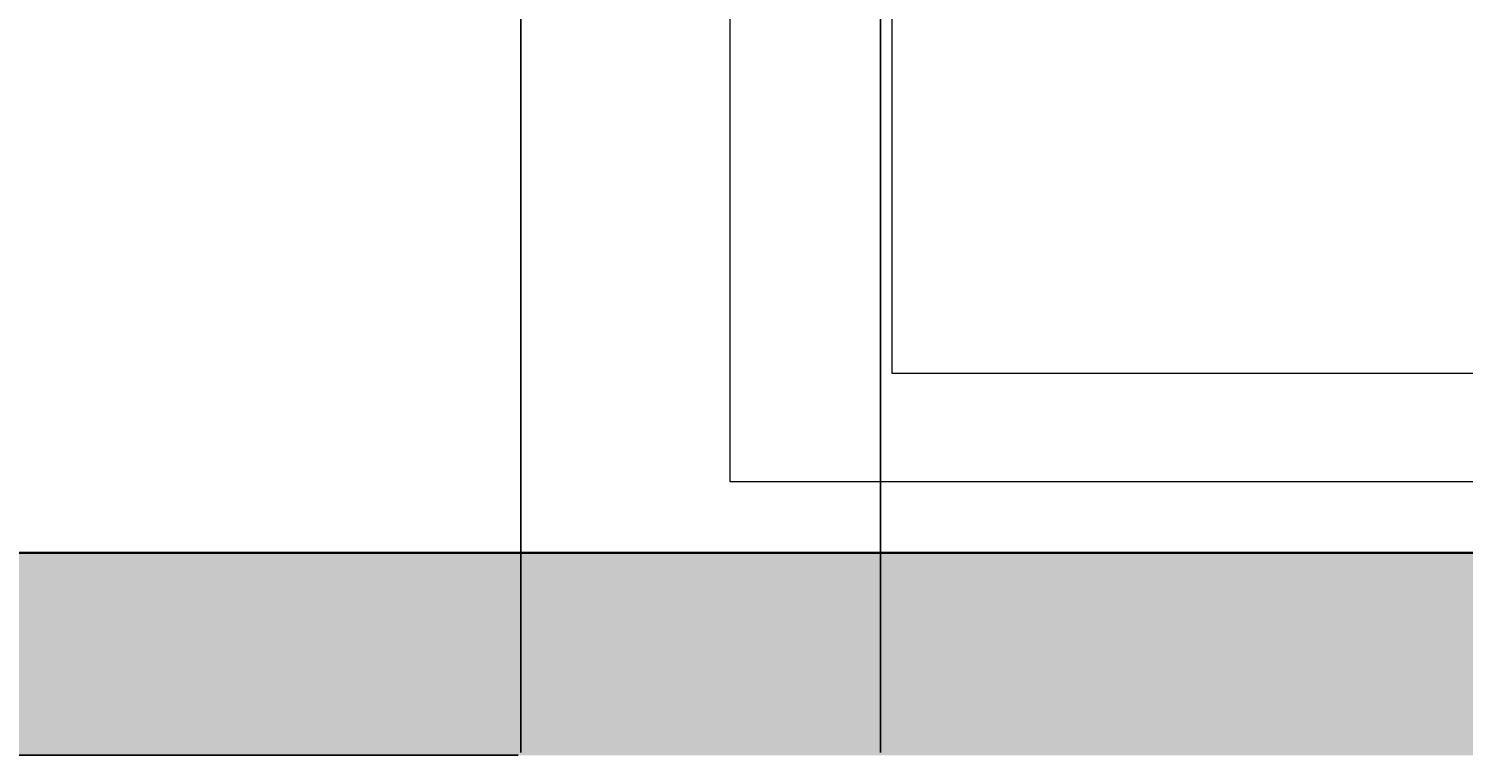
# Model space of a CAD drawing. Units: inches. Extents: x 1998 to 2588, y 1139 to 1977.
# Tile 123 of 134: x 2397 to 2429, y 1637 to 1653. Entities that reach past the tile are written whole.
import ezdxf

# ---------------------------------------------------------------- set-up
doc = ezdxf.new("R2010")
doc.units = ezdxf.units.IN
for name, color, linetype, lineweight in [('A-ANNO-DIMS', 2, 'Continuous', 18), ('A-WALL-PATT', 252, 'Continuous', 13), ('FUR', 21, 'Continuous', 18), ('WALL', 200, 'Continuous', 35)]:
    doc.layers.add(name, color=color, linetype=linetype, lineweight=lineweight)
doc.styles.get("Standard").update_dxf_attribs({"font": 'arial.ttf'})
doc.dimstyles.get("Standard").update_dxf_attribs({"dimtxt": 0.18, "dimasz": 0.18, "dimexe": 0.18, "dimexo": 0.0625, "dimgap": 0.09, "dimtad": 0, "dimtih": 1, "dimtoh": 1, "dimdec": 4, "dimzin": 0, "dimdsep": 46, "dimtxsty": 'Standard', "dimcen": 0.09, "dimadec": 0, "dimazin": 0, "dimtfac": 1, "dimtdec": 4, "dimtofl": 0, "dimtmove": 0, "dimatfit": 3, "dimfxl": 1, "dimtolj": 1, "dimtzin": 0, "dimarcsym": 0})

# ---------------------------------------------------------------- blocks, each defined once
blk = doc.blocks.new('SOFA-THREE-SEAT')
for p, q in [((0, 25.615), (0, 0)), ((0, 0), (74.336, 0))]:
    blk.add_line(p, q)
blk.add_lwpolyline([(3.604, 2.416), (71.008, 2.416), (71.008, 25.615), (3.604, 25.615)], close=True)
blk = doc.blocks.new('*D24')
at = {"layer": 'A-ANNO-DIMS', "color": 0, "lineweight": -2, "transparency": 16777216}
for p, q in [((2398.535, 1911.232), (2588.309, 1911.232)), ((2588.129, 1911.052), (2588.129, 1570.164)), ((2588.129, 1228.912), (2588.129, 1569.8)), ((2527.535, 1228.732), (2588.309, 1228.732))]:
    blk.add_line(p, q, dxfattribs=at)
at = {"layer": 'A-ANNO-DIMS', "color": 0, "transparency": 16777216}
for points in [[(2588.099, 1911.052), (2588.159, 1911.052), (2588.129, 1911.232)], [(2588.099, 1228.912), (2588.159, 1228.912), (2588.129, 1228.732)]]:
    blk.add_solid(points, dxfattribs=at)
at = {"layer": 'Defpoints', "color": 0, "transparency": 16777216}
for p in [(2398.473, 1911.232), (2588.129, 1911.232), (2527.473, 1228.732)]:
    blk.add_point(p, dxfattribs=at)
at = {"layer": 'A-ANNO-DIMS', "color": 0, "transparency": 16777216, "insert": (2588.129, 1569.982), "char_height": 0.18, "attachment_point": 5}
blk.add_mtext('\\A1;682.5', dxfattribs=at)
blk = doc.blocks.new('*D30')
at = {"layer": 'A-ANNO-DIMS', "color": 0, "lineweight": -2, "transparency": 16777216}
for p, q in [((2407.91, 1636.732), (1997.843, 1636.732)), ((1998.023, 1636.552), (1998.023, 1615.913)), ((1998.023, 1594.912), (1998.023, 1615.552)), ((2407.91, 1594.732), (1997.843, 1594.732))]:
    blk.add_line(p, q, dxfattribs=at)
at = {"layer": 'A-ANNO-DIMS', "color": 0, "transparency": 16777216}
for points in [[(1997.993, 1636.552), (1998.053, 1636.552), (1998.023, 1636.732)], [(1997.993, 1594.912), (1998.053, 1594.912), (1998.023, 1594.732)]]:
    blk.add_solid(points, dxfattribs=at)
at = {"layer": 'Defpoints', "color": 0, "transparency": 16777216}
for p in [(1998.023, 1636.732), (2407.973, 1636.732), (2407.973, 1594.732)]:
    blk.add_point(p, dxfattribs=at)
at = {"layer": 'A-ANNO-DIMS', "color": 0, "transparency": 16777216, "insert": (1998.023, 1615.732), "char_height": 0.18, "attachment_point": 5}
blk.add_mtext('\\A1;42', dxfattribs=at)
blk = doc.blocks.new('*D32')
at = {"layer": 'A-ANNO-DIMS', "color": 0, "lineweight": -2, "transparency": 16777216}
for p, q in [((2407.973, 1636.795), (2407.973, 1977.362)), ((2415.973, 1636.795), (2415.973, 1977.362)), ((2408.153, 1977.182), (2411.824, 1977.182)), ((2415.793, 1977.182), (2412.122, 1977.182))]:
    blk.add_line(p, q, dxfattribs=at)
at = {"layer": 'A-ANNO-DIMS', "color": 0, "transparency": 16777216}
for points in [[(2408.153, 1977.212), (2408.153, 1977.152), (2407.973, 1977.182)], [(2415.793, 1977.212), (2415.793, 1977.152), (2415.973, 1977.182)]]:
    blk.add_solid(points, dxfattribs=at)
at = {"layer": 'Defpoints', "color": 0, "transparency": 16777216}
for p in [(2415.973, 1977.182), (2407.973, 1636.732), (2415.973, 1636.732)]:
    blk.add_point(p, dxfattribs=at)
at = {"layer": 'A-ANNO-DIMS', "color": 0, "transparency": 16777216, "insert": (2411.973, 1977.182), "char_height": 0.18, "attachment_point": 5}
blk.add_mtext('\\A1;8', dxfattribs=at)

msp = doc.modelspace()

# ---------------------------------------------------------------- hatches: boundary and pattern name
at = {"layer": 'A-WALL-PATT'}
h = msp.add_hatch(color=256, dxfattribs=at)
h.dxf.hatch_style = 1
h.paths.add_polyline_path([(2527.4729, 1362.2324), (2510.9729, 1362.2324), (2510.9729, 1357.7324), (2518.4729, 1357.7324), (2518.4729, 1237.7324), (2503.1458, 1237.7324), (2503.1458, 1228.7324), (2527.4729, 1228.7324)])
h.paths.add_polyline_path([(2490.5682, 1362.2324), (2398.4729, 1362.2324), (2398.4729, 1357.7324), (2490.5682, 1357.7324)])
h.paths.add_polyline_path([(2224.9729, 1264.7324), (2222.9729, 1264.7324), (2222.9729, 1232.4125), (2341.4729, 1232.4125), (2341.4729, 1234.4125), (2224.9729, 1234.4125)])
h.paths.add_polyline_path([(2334.5332, 1273.7324), (2264.7638, 1273.7324), (2264.7638, 1269.5611, -0.043659), (2264.3413, 1264.7324), (2334.5332, 1264.7324)])
h.paths.add_polyline_path([(2236.9551, 1273.7324), (2234.4125, 1273.7324), (2234.4125, 1264.7324), (2236.9551, 1264.7324), (2236.9551, 1269.5611)])
h.paths.add_polyline_path([(2222.9729, 1293.2324), (2096.9729, 1293.2324), (2096.9729, 1345.0966), (2087.9729, 1345.0966), (2087.9729, 1284.2324), (2222.9729, 1284.2324), (2222.9729, 1285.137)])
h.paths.add_polyline_path([(2096.9729, 1458.7927), (2087.9729, 1458.7927), (2087.9729, 1417.7324), (2087.9729, 1413.2324), (2096.9729, 1413.2324), (2096.9729, 1417.7324)])
h.paths.add_polyline_path([(2096.9729, 1413.2324), (2087.9729, 1413.2324), (2087.9729, 1365.5012), (2096.9729, 1365.5012), (2096.9729, 1369.3358)])
h.paths.add_polyline_path([(2186.2943, 1417.7324), (2138.6074, 1417.7324), (2096.9729, 1417.7324), (2096.9729, 1413.2324), (2138.6074, 1413.2324), (2186.2943, 1413.2324)])
h.paths.add_polyline_path([(2181.4729, 1465.7324), (2176.9729, 1465.7324), (2176.9729, 1451.6434), (2181.4729, 1451.6434)])
h.paths.add_polyline_path([(2181.4729, 1422.1664), (2176.9729, 1422.1664), (2176.9729, 1417.7324), (2181.4729, 1417.7324)])
h.paths.add_polyline_path([(2063.9729, 1465.7324), (2087.9729, 1465.7324), (2087.9729, 1470.2324), (2059.4729, 1470.2324), (2059.4729, 1413.2324), (2087.9729, 1413.2324), (2087.9729, 1417.7324), (2063.9729, 1417.7324)])
h.paths.add_polyline_path([(2181.4729, 1755.2324), (2176.9729, 1755.2324), (2176.9729, 1748.6798), (2177.0513, 1748.6798), (2181.4729, 1748.6798)])
h.paths.add_polyline_path([(2227.4729, 1707.2324), (2220.4647, 1707.2324), (2220.4647, 1702.7324), (2222.9729, 1702.7324), (2222.9729, 1604.637), (2227.4729, 1604.637)])
h.paths.add_polyline_path([(2114.9729, 1702.7324), (2105.9729, 1702.7324), (2105.9729, 1628.4781, -0.0318759), (2110.1012, 1628.7416), (2114.9729, 1628.7416)])
h.paths.add_polyline_path([(2345.9729, 1739.3278), (2341.4729, 1739.3278), (2341.4729, 1647.5211), (2345.9729, 1647.5211)])
h.paths.add_polyline_path([(2350.6273, 1641.2324), (2345.9729, 1641.2324), (2345.9729, 1636.7324), (2350.6273, 1636.7324), (2350.6273, 1639.8729)])
h.paths.add_polyline_path([(2501.9729, 1641.2324), (2407.9729, 1641.2324), (2392.5005, 1641.2324), (2392.5005, 1639.8729), (2392.5005, 1636.7324), (2501.9729, 1636.7324)])
h.paths.add_polyline_path([(2510.9729, 1755.2324), (2501.9729, 1755.2324), (2501.9729, 1641.2324), (2510.9729, 1641.2324)])
h.paths.add_polyline_path([(2549.1786, 1641.2324), (2522.3775, 1641.2324), (2522.3775, 1636.7324), (2540.1786, 1636.7324), (2540.1786, 1480.7324), (2522.3775, 1480.7324), (2522.3775, 1476.2324), (2549.1786, 1476.2324)])
h.paths.add_polyline_path([(2498.1786, 1594.7324), (2407.9729, 1594.7324), (2407.9729, 1585.7324), (2416.9729, 1585.7324), (2489.1786, 1585.7324), (2489.1786, 1531.7324), (2416.9729, 1531.7324), (2407.9729, 1531.7324), (2407.9729, 1522.7324), (2498.1786, 1522.7324)])
h.paths.add_polyline_path([(2351.6437, 1480.7324), (2345.9729, 1480.7324), (2345.9729, 1476.2324), (2351.6437, 1476.2324), (2351.6437, 1477.5919)])
h.paths.add_polyline_path([(2501.9729, 1480.7324), (2498.1786, 1480.7324), (2407.9729, 1480.7324), (2393.5168, 1480.7324), (2393.5168, 1477.5919), (2393.5168, 1476.2324), (2501.9729, 1476.2324)])

# ---------------------------------------------------------------- linework, layer by layer
at = {"layer": 'WALL'}
for p, q in [((2501.9729, 1641.2324), (2391.5845, 1641.2324)), ((2407.9729, 1641.2324), (2549.1786, 1641.2324))]:
    msp.add_line(p, q, dxfattribs=at)

# ---------------------------------------------------------------- block references
at = {"layer": 'FUR'}
msp.add_blockref('SOFA-THREE-SEAT', (2412.6207, 1642.8172), dxfattribs=at)

# ---------------------------------------------------------------- dimensions: what is measured, and where the dimension line sits
at = {"layer": 'A-ANNO-DIMS'}
dim = msp.add_linear_dim(base=(2415.9729, 1977.1824), p1=(2407.9729, 1636.7324), p2=(2415.9729, 1636.7324), dimstyle='Standard', override={"dimdec": 0, "dimlfac": 1, "dimrnd": 0, "dimzin": 0, "dimdsep": 46, "dimlunit": 2}, dxfattribs=at)
dim.commit()
dim.dimension.update_dxf_attribs({"geometry": '*D32', "text_midpoint": (2411.9729, 1977.1824)})
for base, p1, p2, override, picture, middle in [((2588.1286, 1911.2324), (2527.4729, 1228.7324), (2398.4729, 1911.2324), {"dimdec": 1, "dimlfac": 1, "dimrnd": 0, "dimzin": 0, "dimdsep": 46, "dimlunit": 2}, '*D24', (2588.1286, 1569.9824)), ((1998.0229, 1636.7324), (2407.9729, 1594.7324), (2407.9729, 1636.7324), {"dimdec": 0, "dimlfac": 1, "dimrnd": 0, "dimzin": 0, "dimdsep": 46, "dimlunit": 2}, '*D30', (1998.0229, 1615.7324))]:
    dim = msp.add_linear_dim(base=base, p1=p1, p2=p2, angle=90, dimstyle='Standard', override=override, dxfattribs=at)
    dim.commit()
    dim.dimension.update_dxf_attribs({"geometry": picture, "text_midpoint": middle})

doc.saveas('drawing.dxf')
